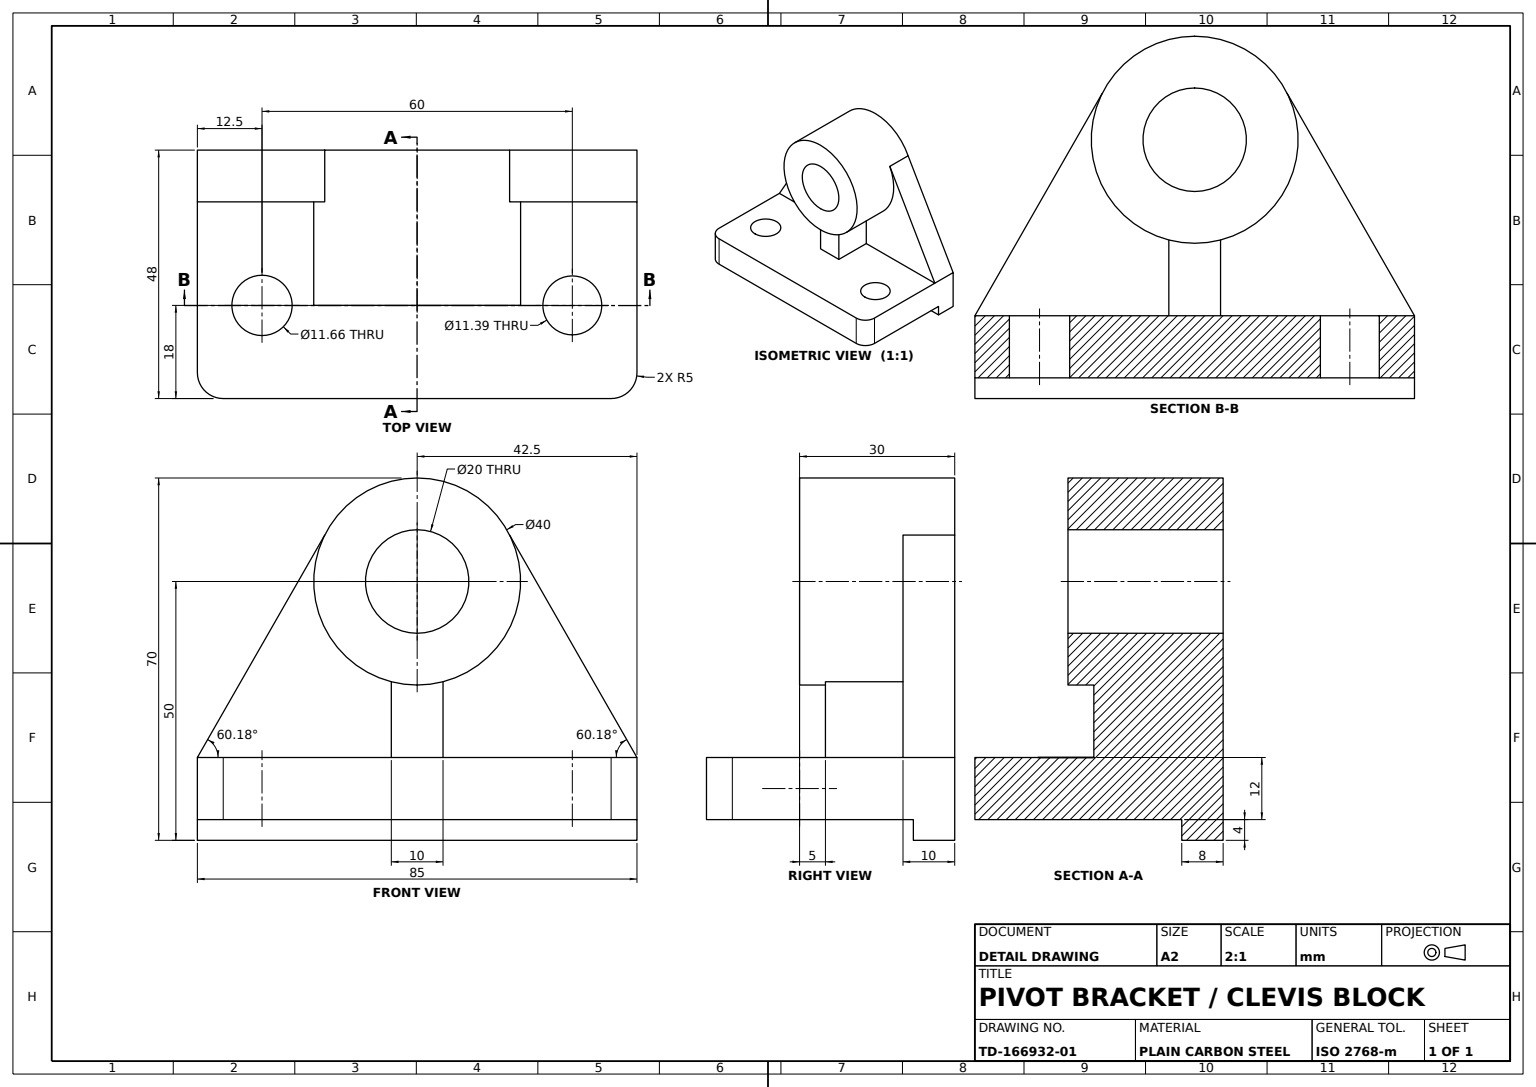
SolidWorks part; units mm, degrees
material "Plain Carbon Steel"
ref_plane "Front Plane" through (0, 0, 0) normal (0, 0, 1) x (1, 0, 0)
ref_plane "Top Plane" through (0, 0, 0) normal (0, 1, 0) x (1, 0, 0)
ref_plane "Right Plane" through (0, 0, 0) normal (1, 0, 0) x (0, 0, -1)
sketch "Base Plate Profile Sketch" plane through (0, 0, 0) normal (0, 0, 1) x (1, 0, 0)
  line L0 (0, 0) -> (0, 16)
  line L1 (0, 16) -> (48, 16)
  line L2 (48, 16) -> (48, 4)
  line L3 (48, 4) -> (8, 4)
  line L4 (8, 4) -> (8, 0)
  line L5 (8, 0) -> (0, 0)
  dimension "D1" = 48
  dimension "D2" = 4
  dimension "D3" = 12
  dimension "D4" = 8
extrude "Base Plate" add sketch "Base Plate Profile Sketch" along normal blind 85
sketch "Pivot Boss Sketch" plane through (0, 0, 0) normal (-1, 0, 0) x (0, 0, 1)
  line L0 (85, 0) -> (0, 0) construction
  line L1 (0, 16) -> (0, 0) construction
  circle A0 centre (42.5, 50) radius 20
  dimension "D2" = 40
  dimension "D1" = 50
  dimension "D3" = 42.5
extrude "Pivot Boss" add sketch "Pivot Boss Sketch" against normal blind 30 separate body
sketch "Gusset Rib Sketch" plane through (0, 0, 0) normal (-1, 0, 0) x (0, 0, 1)
  line L0 (0, 16) -> (25.7214, 60.8848)
  line L1 (85, 16) -> (59.2786, 60.8848)
  line L2 (0, 16) -> (85, 16)
  circle A0 centre (42.5, 50) radius 20 construction
  circle A2 centre (42.5, 50) radius 20
  arc A3 (25.7214, 60.8848) -> (59.2786, 60.8848) centre (42.5, 50) ccw
  circle M3 centre (42.5, 50) radius 20
  dimension "D1" = 51.7323
  dimension "D3" = 16.7786
  dimension "D2" = 0
extrude "Gusset Rib" add sketch "Gusset Rib Sketch" against normal blind 10 contours L0 L2 L1 M3
sketch "Boss Support Block Sketch" plane through (0, 16, 0) normal (0, 1, 0) x (1, 0, 0)
  line L0 (10, 0) -> (10, -85) construction
  line L1 (10, -37.5) -> (25, -37.5)
  line L2 (10, -37.5) -> (10, -47.5)
  line L3 (10, -47.5) -> (25, -47.5)
  line L4 (25, -37.5) -> (25, -47.5)
  line L5 (0, -24.6259) -> (0, -60.3741) construction
  point P8 (0, -42.5)
  dimension "D1" = 5
  dimension "D2" = 5
  dimension "D3" = 15
extrude "Boss Support Block" add sketch "Boss Support Block Sketch" along normal up to surface up to face at (30, 30, 42.5)
sketch "Pivot Bore Sketch" plane through (30, 0, 0) normal (1, 0, 0) x (0, 0, -1)
  circle A0 centre (-42.5, 50) radius 10
  dimension "D1" = 20
extrude "Pivot Bore Ø20" cut sketch "Pivot Bore Sketch" against normal through all
sketch "Mounting Holes Sketch" plane through (0, 16, 0) normal (0, 1, 0) x (1, 0, 0)
  line L0 (48, 0) -> (10, 0) construction
  line L3 (48, -85) -> (48, 0) construction
  circle A0 centre (30, -12.5) radius 5.6971
  circle A1 centre (30, -72.5) radius 5.8295
  dimension "D4" = 11.6591
  dimension "D5" = 11.3941
  dimension "D1" = 60
  dimension "D2" = 12.5
  dimension "D3" = 18
extrude "Mounting Holes 2x" cut sketch "Mounting Holes Sketch" against normal through all
fillet "Corner Fillets R5" radius 5 2 edges at (48, 10, 0) (48, 10, 85)
